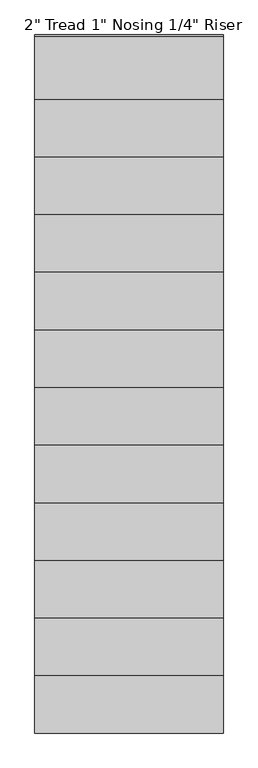
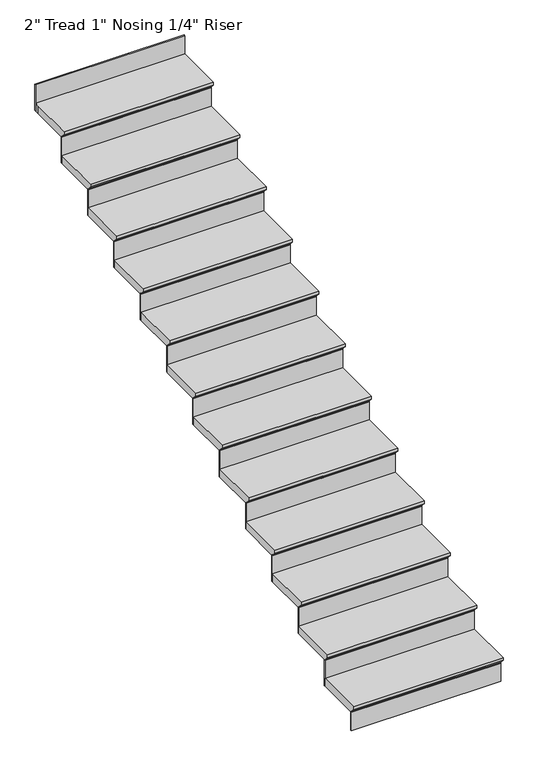
"""IFC4 building model written with IfcOpenShell, lengths in millimetres: stair flight geometry."""

from ifc_helpers import new_model, si_unit, origin, place, context, project, spatial, faceted_brep, source, transform, mapped, element, save


def stair_flight_74cd6fce(model_context):
    return source(origin(), model_context, "Body", "Brep", [
        faceted_brep([(-2703.0415084, 19841.9216096, 34528.9005799), (-2703.0415084, 19841.9216096, 34547.9505799), (-3617.4415084, 19841.9216096, 34547.9505799), (-3617.4415084, 19841.9216096, 34528.9005799), (-2703.0415084, 19867.3216096, 34503.5005799), (-3617.4415084, 19867.3216096, 34503.5005799), (-2703.0415084, 20146.7216096, 34547.9505799), (-3617.4415084, 20146.7216096, 34547.9505799), (-3617.4415084, 19867.3216096, 34497.1505799), (-3617.4415084, 20146.7216096, 34497.1505799), (-2703.0415084, 20146.7216096, 34497.1505799), (-2703.0415084, 19867.3216096, 34497.1505799)], [[[0, 1, 2, 3]], [[4, 0, 3, 5]], [[2, 1, 6, 7]], [[8, 9, 10, 11]], [[2, 7, 9, 8, 5, 3]], [[8, 11, 4, 5]], [[6, 1, 0, 4, 11, 10]], [[7, 6, 10, 9]]]),
        faceted_brep([(-2703.0415084, 19867.3216096, 34497.1505799), (-2703.0415084, 19867.3216096, 34378.6172466), (-2703.0415084, 19873.6716096, 34378.6172466), (-2703.0415084, 19873.6716096, 34497.1505799), (-3617.4415084, 19867.3216096, 34497.1505799), (-3617.4415084, 19873.6716096, 34497.1505799), (-3617.4415084, 19873.6716096, 34378.6172466), (-3617.4415084, 19867.3216096, 34378.6172466)], [[[0, 1, 2, 3]], [[4, 5, 6, 7]], [[1, 0, 4, 7]], [[2, 1, 7, 6]], [[3, 2, 6, 5]], [[0, 3, 5, 4]]]),
        faceted_brep([(-2703.0415084, 20146.7216096, 34666.4839133), (-2703.0415084, 20146.7216096, 34497.1505799), (-2703.0415084, 20153.0716096, 34497.1505799), (-2703.0415084, 20153.0716096, 34666.4839133), (-3617.4415084, 20146.7216096, 34666.4839133), (-3617.4415084, 20153.0716096, 34666.4839133), (-3617.4415084, 20153.0716096, 34497.1505799), (-3617.4415084, 20146.7216096, 34497.1505799)], [[[0, 1, 2, 3]], [[4, 5, 6, 7]], [[1, 0, 4, 7]], [[2, 1, 7, 6]], [[3, 2, 6, 5]], [[0, 3, 5, 4]]]),
        faceted_brep([(-3617.4415084, 20121.3216096, 34717.2839133), (-2703.0415084, 20121.3216096, 34717.2839133), (-2703.0415084, 20426.1216096, 34717.2839133), (-3617.4415084, 20426.1216096, 34717.2839133), (-3617.4415084, 20146.7216096, 34666.4839133), (-3617.4415084, 20426.1216096, 34666.4839133), (-2703.0415084, 20426.1216096, 34666.4839133), (-2703.0415084, 20146.7216096, 34666.4839133), (-3617.4415084, 20146.7216096, 34672.8339133), (-3617.4415084, 20121.3216096, 34698.2339133), (-2703.0415084, 20146.7216096, 34672.8339133), (-2703.0415084, 20121.3216096, 34698.2339133)], [[[0, 1, 2, 3]], [[4, 5, 6, 7]], [[0, 3, 5, 4, 8, 9]], [[4, 7, 10, 8]], [[2, 1, 11, 10, 7, 6]], [[3, 2, 6, 5]], [[11, 1, 0, 9]], [[10, 11, 9, 8]]]),
        faceted_brep([(-2703.0415084, 20426.1216096, 34835.8172466), (-2703.0415084, 20426.1216096, 34666.4839133), (-2703.0415084, 20432.4716096, 34666.4839133), (-2703.0415084, 20432.4716096, 34835.8172466), (-3617.4415084, 20426.1216096, 34835.8172466), (-3617.4415084, 20432.4716096, 34835.8172466), (-3617.4415084, 20432.4716096, 34666.4839133), (-3617.4415084, 20426.1216096, 34666.4839133)], [[[0, 1, 2, 3]], [[4, 5, 6, 7]], [[1, 0, 4, 7]], [[2, 1, 7, 6]], [[3, 2, 6, 5]], [[0, 3, 5, 4]]]),
        faceted_brep([(-3617.4415084, 20400.7216096, 34886.6172466), (-2703.0415084, 20400.7216096, 34886.6172466), (-2703.0415084, 20705.5216096, 34886.6172466), (-3617.4415084, 20705.5216096, 34886.6172466), (-3617.4415084, 20426.1216096, 34835.8172466), (-3617.4415084, 20705.5216096, 34835.8172466), (-2703.0415084, 20705.5216096, 34835.8172466), (-2703.0415084, 20426.1216096, 34835.8172466), (-3617.4415084, 20426.1216096, 34842.1672466), (-3617.4415084, 20400.7216096, 34867.5672466), (-2703.0415084, 20426.1216096, 34842.1672466), (-2703.0415084, 20400.7216096, 34867.5672466)], [[[0, 1, 2, 3]], [[4, 5, 6, 7]], [[0, 3, 5, 4, 8, 9]], [[4, 7, 10, 8]], [[2, 1, 11, 10, 7, 6]], [[3, 2, 6, 5]], [[11, 1, 0, 9]], [[10, 11, 9, 8]]]),
        faceted_brep([(-2703.0415084, 20705.5216096, 35005.1505799), (-2703.0415084, 20705.5216096, 34835.8172466), (-2703.0415084, 20711.8716096, 34835.8172466), (-2703.0415084, 20711.8716096, 35005.1505799), (-3617.4415084, 20705.5216096, 35005.1505799), (-3617.4415084, 20711.8716096, 35005.1505799), (-3617.4415084, 20711.8716096, 34835.8172466), (-3617.4415084, 20705.5216096, 34835.8172466)], [[[0, 1, 2, 3]], [[4, 5, 6, 7]], [[1, 0, 4, 7]], [[2, 1, 7, 6]], [[3, 2, 6, 5]], [[0, 3, 5, 4]]]),
        faceted_brep([(-3617.4415084, 20680.1216096, 35055.9505799), (-2703.0415084, 20680.1216096, 35055.9505799), (-2703.0415084, 20984.9216096, 35055.9505799), (-3617.4415084, 20984.9216096, 35055.9505799), (-3617.4415084, 20705.5216096, 35005.1505799), (-3617.4415084, 20984.9216096, 35005.1505799), (-2703.0415084, 20984.9216096, 35005.1505799), (-2703.0415084, 20705.5216096, 35005.1505799), (-3617.4415084, 20705.5216096, 35011.5005799), (-3617.4415084, 20680.1216096, 35036.9005799), (-2703.0415084, 20705.5216096, 35011.5005799), (-2703.0415084, 20680.1216096, 35036.9005799)], [[[0, 1, 2, 3]], [[4, 5, 6, 7]], [[0, 3, 5, 4, 8, 9]], [[4, 7, 10, 8]], [[2, 1, 11, 10, 7, 6]], [[3, 2, 6, 5]], [[11, 1, 0, 9]], [[10, 11, 9, 8]]]),
        faceted_brep([(-2703.0415084, 20984.9216096, 35174.4839133), (-2703.0415084, 20984.9216096, 35005.1505799), (-2703.0415084, 20991.2716096, 35005.1505799), (-2703.0415084, 20991.2716096, 35174.4839133), (-3617.4415084, 20984.9216096, 35174.4839133), (-3617.4415084, 20991.2716096, 35174.4839133), (-3617.4415084, 20991.2716096, 35005.1505799), (-3617.4415084, 20984.9216096, 35005.1505799)], [[[0, 1, 2, 3]], [[4, 5, 6, 7]], [[1, 0, 4, 7]], [[2, 1, 7, 6]], [[3, 2, 6, 5]], [[0, 3, 5, 4]]]),
        faceted_brep([(-3617.4415084, 20959.5216096, 35225.2839133), (-2703.0415084, 20959.5216096, 35225.2839133), (-2703.0415084, 21264.3216096, 35225.2839133), (-3617.4415084, 21264.3216096, 35225.2839133), (-3617.4415084, 20984.9216096, 35174.4839133), (-3617.4415084, 21264.3216096, 35174.4839133), (-2703.0415084, 21264.3216096, 35174.4839133), (-2703.0415084, 20984.9216096, 35174.4839133), (-3617.4415084, 20984.9216096, 35180.8339133), (-3617.4415084, 20959.5216096, 35206.2339133), (-2703.0415084, 20984.9216096, 35180.8339133), (-2703.0415084, 20959.5216096, 35206.2339133)], [[[0, 1, 2, 3]], [[4, 5, 6, 7]], [[0, 3, 5, 4, 8, 9]], [[4, 7, 10, 8]], [[2, 1, 11, 10, 7, 6]], [[3, 2, 6, 5]], [[11, 1, 0, 9]], [[10, 11, 9, 8]]]),
        faceted_brep([(-2703.0415084, 21264.3216096, 35343.8172466), (-2703.0415084, 21264.3216096, 35174.4839133), (-2703.0415084, 21270.6716096, 35174.4839133), (-2703.0415084, 21270.6716096, 35343.8172466), (-3617.4415084, 21264.3216096, 35343.8172466), (-3617.4415084, 21270.6716096, 35343.8172466), (-3617.4415084, 21270.6716096, 35174.4839133), (-3617.4415084, 21264.3216096, 35174.4839133)], [[[0, 1, 2, 3]], [[4, 5, 6, 7]], [[1, 0, 4, 7]], [[2, 1, 7, 6]], [[3, 2, 6, 5]], [[0, 3, 5, 4]]]),
        faceted_brep([(-3617.4415084, 21238.9216096, 35394.6172466), (-2703.0415084, 21238.9216096, 35394.6172466), (-2703.0415084, 21543.7216096, 35394.6172466), (-3617.4415084, 21543.7216096, 35394.6172466), (-3617.4415084, 21264.3216096, 35343.8172466), (-3617.4415084, 21543.7216096, 35343.8172466), (-2703.0415084, 21543.7216096, 35343.8172466), (-2703.0415084, 21264.3216096, 35343.8172466), (-3617.4415084, 21264.3216096, 35350.1672466), (-3617.4415084, 21238.9216096, 35375.5672466), (-2703.0415084, 21264.3216096, 35350.1672466), (-2703.0415084, 21238.9216096, 35375.5672466)], [[[0, 1, 2, 3]], [[4, 5, 6, 7]], [[0, 3, 5, 4, 8, 9]], [[4, 7, 10, 8]], [[2, 1, 11, 10, 7, 6]], [[3, 2, 6, 5]], [[11, 1, 0, 9]], [[10, 11, 9, 8]]]),
        faceted_brep([(-2703.0415084, 21543.7216096, 35513.1505799), (-2703.0415084, 21543.7216096, 35343.8172466), (-2703.0415084, 21550.0716096, 35343.8172466), (-2703.0415084, 21550.0716096, 35513.1505799), (-3617.4415084, 21543.7216096, 35513.1505799), (-3617.4415084, 21550.0716096, 35513.1505799), (-3617.4415084, 21550.0716096, 35343.8172466), (-3617.4415084, 21543.7216096, 35343.8172466)], [[[0, 1, 2, 3]], [[4, 5, 6, 7]], [[1, 0, 4, 7]], [[2, 1, 7, 6]], [[3, 2, 6, 5]], [[0, 3, 5, 4]]]),
        faceted_brep([(-3617.4415084, 21518.3216096, 35563.9505799), (-2703.0415084, 21518.3216096, 35563.9505799), (-2703.0415084, 21823.1216096, 35563.9505799), (-3617.4415084, 21823.1216096, 35563.9505799), (-3617.4415084, 21543.7216096, 35513.1505799), (-3617.4415084, 21823.1216096, 35513.1505799), (-2703.0415084, 21823.1216096, 35513.1505799), (-2703.0415084, 21543.7216096, 35513.1505799), (-3617.4415084, 21543.7216096, 35519.5005799), (-3617.4415084, 21518.3216096, 35544.9005799), (-2703.0415084, 21543.7216096, 35519.5005799), (-2703.0415084, 21518.3216096, 35544.9005799)], [[[0, 1, 2, 3]], [[4, 5, 6, 7]], [[0, 3, 5, 4, 8, 9]], [[4, 7, 10, 8]], [[2, 1, 11, 10, 7, 6]], [[3, 2, 6, 5]], [[11, 1, 0, 9]], [[10, 11, 9, 8]]]),
        faceted_brep([(-2703.0415084, 21823.1216096, 35682.4839133), (-2703.0415084, 21823.1216096, 35513.1505799), (-2703.0415084, 21829.4716096, 35513.1505799), (-2703.0415084, 21829.4716096, 35682.4839133), (-3617.4415084, 21823.1216096, 35682.4839133), (-3617.4415084, 21829.4716096, 35682.4839133), (-3617.4415084, 21829.4716096, 35513.1505799), (-3617.4415084, 21823.1216096, 35513.1505799)], [[[0, 1, 2, 3]], [[4, 5, 6, 7]], [[1, 0, 4, 7]], [[2, 1, 7, 6]], [[3, 2, 6, 5]], [[0, 3, 5, 4]]]),
        faceted_brep([(-3617.4415084, 21797.7216096, 35733.2839133), (-2703.0415084, 21797.7216096, 35733.2839133), (-2703.0415084, 22102.5216096, 35733.2839133), (-3617.4415084, 22102.5216096, 35733.2839133), (-3617.4415084, 21823.1216096, 35682.4839133), (-3617.4415084, 22102.5216096, 35682.4839133), (-2703.0415084, 22102.5216096, 35682.4839133), (-2703.0415084, 21823.1216096, 35682.4839133), (-3617.4415084, 21823.1216096, 35688.8339133), (-3617.4415084, 21797.7216096, 35714.2339133), (-2703.0415084, 21823.1216096, 35688.8339133), (-2703.0415084, 21797.7216096, 35714.2339133)], [[[0, 1, 2, 3]], [[4, 5, 6, 7]], [[0, 3, 5, 4, 8, 9]], [[4, 7, 10, 8]], [[2, 1, 11, 10, 7, 6]], [[3, 2, 6, 5]], [[11, 1, 0, 9]], [[10, 11, 9, 8]]]),
        faceted_brep([(-2703.0415084, 22102.5216096, 35851.8172466), (-2703.0415084, 22102.5216096, 35682.4839133), (-2703.0415084, 22108.8716096, 35682.4839133), (-2703.0415084, 22108.8716096, 35851.8172466), (-3617.4415084, 22102.5216096, 35851.8172466), (-3617.4415084, 22108.8716096, 35851.8172466), (-3617.4415084, 22108.8716096, 35682.4839133), (-3617.4415084, 22102.5216096, 35682.4839133)], [[[0, 1, 2, 3]], [[4, 5, 6, 7]], [[1, 0, 4, 7]], [[2, 1, 7, 6]], [[3, 2, 6, 5]], [[0, 3, 5, 4]]]),
        faceted_brep([(-3617.4415084, 22077.1216096, 35902.6172466), (-2703.0415084, 22077.1216096, 35902.6172466), (-2703.0415084, 22381.9216096, 35902.6172466), (-3617.4415084, 22381.9216096, 35902.6172466), (-3617.4415084, 22102.5216096, 35851.8172466), (-3617.4415084, 22381.9216096, 35851.8172466), (-2703.0415084, 22381.9216096, 35851.8172466), (-2703.0415084, 22102.5216096, 35851.8172466), (-3617.4415084, 22102.5216096, 35858.1672466), (-3617.4415084, 22077.1216096, 35883.5672466), (-2703.0415084, 22102.5216096, 35858.1672466), (-2703.0415084, 22077.1216096, 35883.5672466)], [[[0, 1, 2, 3]], [[4, 5, 6, 7]], [[0, 3, 5, 4, 8, 9]], [[4, 7, 10, 8]], [[2, 1, 11, 10, 7, 6]], [[3, 2, 6, 5]], [[11, 1, 0, 9]], [[10, 11, 9, 8]]]),
        faceted_brep([(-2703.0415084, 22381.9216096, 36021.1505799), (-2703.0415084, 22381.9216096, 35851.8172466), (-2703.0415084, 22388.2716096, 35851.8172466), (-2703.0415084, 22388.2716096, 36021.1505799), (-3617.4415084, 22381.9216096, 36021.1505799), (-3617.4415084, 22388.2716096, 36021.1505799), (-3617.4415084, 22388.2716096, 35851.8172466), (-3617.4415084, 22381.9216096, 35851.8172466)], [[[0, 1, 2, 3]], [[4, 5, 6, 7]], [[1, 0, 4, 7]], [[2, 1, 7, 6]], [[3, 2, 6, 5]], [[0, 3, 5, 4]]]),
        faceted_brep([(-3617.4415084, 22356.5216096, 36071.9505799), (-2703.0415084, 22356.5216096, 36071.9505799), (-2703.0415084, 22661.3216096, 36071.9505799), (-3617.4415084, 22661.3216096, 36071.9505799), (-3617.4415084, 22381.9216096, 36021.1505799), (-3617.4415084, 22661.3216096, 36021.1505799), (-2703.0415084, 22661.3216096, 36021.1505799), (-2703.0415084, 22381.9216096, 36021.1505799), (-3617.4415084, 22381.9216096, 36027.5005799), (-3617.4415084, 22356.5216096, 36052.9005799), (-2703.0415084, 22381.9216096, 36027.5005799), (-2703.0415084, 22356.5216096, 36052.9005799)], [[[0, 1, 2, 3]], [[4, 5, 6, 7]], [[0, 3, 5, 4, 8, 9]], [[4, 7, 10, 8]], [[2, 1, 11, 10, 7, 6]], [[3, 2, 6, 5]], [[11, 1, 0, 9]], [[10, 11, 9, 8]]]),
        faceted_brep([(-2703.0415084, 22661.3216096, 36190.4839133), (-2703.0415084, 22661.3216096, 36021.1505799), (-2703.0415084, 22667.6716096, 36021.1505799), (-2703.0415084, 22667.6716096, 36190.4839133), (-3617.4415084, 22661.3216096, 36190.4839133), (-3617.4415084, 22667.6716096, 36190.4839133), (-3617.4415084, 22667.6716096, 36021.1505799), (-3617.4415084, 22661.3216096, 36021.1505799)], [[[0, 1, 2, 3]], [[4, 5, 6, 7]], [[1, 0, 4, 7]], [[2, 1, 7, 6]], [[3, 2, 6, 5]], [[0, 3, 5, 4]]]),
        faceted_brep([(-3617.4415084, 22635.9216096, 36241.2839133), (-2703.0415084, 22635.9216096, 36241.2839133), (-2703.0415084, 22940.7216096, 36241.2839133), (-3617.4415084, 22940.7216096, 36241.2839133), (-3617.4415084, 22661.3216096, 36190.4839133), (-3617.4415084, 22940.7216096, 36190.4839133), (-2703.0415084, 22940.7216096, 36190.4839133), (-2703.0415084, 22661.3216096, 36190.4839133), (-3617.4415084, 22661.3216096, 36196.8339133), (-3617.4415084, 22635.9216096, 36222.2339133), (-2703.0415084, 22661.3216096, 36196.8339133), (-2703.0415084, 22635.9216096, 36222.2339133)], [[[0, 1, 2, 3]], [[4, 5, 6, 7]], [[0, 3, 5, 4, 8, 9]], [[4, 7, 10, 8]], [[2, 1, 11, 10, 7, 6]], [[3, 2, 6, 5]], [[11, 1, 0, 9]], [[10, 11, 9, 8]]]),
        faceted_brep([(-2703.0415084, 23220.1216096, 36529.1505799), (-2703.0415084, 23220.1216096, 36359.8172466), (-2703.0415084, 23226.4716096, 36359.8172466), (-2703.0415084, 23226.4716096, 36529.1505799), (-3617.4415084, 23220.1216096, 36529.1505799), (-3617.4415084, 23226.4716096, 36529.1505799), (-3617.4415084, 23226.4716096, 36359.8172466), (-3617.4415084, 23220.1216096, 36359.8172466)], [[[0, 1, 2, 3]], [[4, 5, 6, 7]], [[1, 0, 4, 7]], [[2, 1, 7, 6]], [[3, 2, 6, 5]], [[0, 3, 5, 4]]]),
        faceted_brep([(-2703.0415084, 22940.7216096, 36359.8172466), (-2703.0415084, 22940.7216096, 36190.4839133), (-2703.0415084, 22947.0716096, 36190.4839133), (-2703.0415084, 22947.0716096, 36359.8172466), (-3617.4415084, 22940.7216096, 36359.8172466), (-3617.4415084, 22947.0716096, 36359.8172466), (-3617.4415084, 22947.0716096, 36190.4839133), (-3617.4415084, 22940.7216096, 36190.4839133)], [[[0, 1, 2, 3]], [[4, 5, 6, 7]], [[1, 0, 4, 7]], [[2, 1, 7, 6]], [[3, 2, 6, 5]], [[0, 3, 5, 4]]]),
        faceted_brep([(-3617.4415084, 23220.1216096, 36410.6172466), (-3617.4415084, 23194.7216096, 36410.6172466), (-3617.4415084, 22915.3216096, 36410.6172466), (-2703.0415084, 22915.3216096, 36410.6172466), (-2703.0415084, 23220.1216096, 36410.6172466), (-3617.4415084, 23194.7216096, 36359.8172466), (-3617.4415084, 23220.1216096, 36359.8172466), (-2703.0415084, 23220.1216096, 36359.8172466), (-2703.0415084, 22940.7216096, 36359.8172466), (-3617.4415084, 22940.7216096, 36359.8172466), (-3617.4415084, 22940.7216096, 36366.1672466), (-3617.4415084, 22915.3216096, 36391.5672466), (-2703.0415084, 22940.7216096, 36366.1672466), (-2703.0415084, 22915.3216096, 36391.5672466)], [[[0, 1, 2, 3, 4]], [[5, 6, 7, 8, 9]], [[1, 0, 6, 5]], [[2, 1, 5, 9, 10, 11]], [[9, 8, 12, 10]], [[4, 3, 13, 12, 8, 7]], [[0, 4, 7, 6]], [[13, 3, 2, 11]], [[12, 13, 11, 10]]]),
    ])


if __name__ == "__main__":
    model = new_model("IFC4")
    model_context = context("Model", 3, world=origin())
    ifc_project = project(units=[si_unit("LENGTHUNIT", "METRE", prefix="MILLI")], contexts=[model_context])
    site = spatial("IfcSite", under=ifc_project)
    building = spatial("IfcBuilding", under=site)
    placement = place(None, origin())
    stair_flight_shape = stair_flight_74cd6fce(model_context)
    element("IfcStairFlight", 1, ObjectType="2\" Tread 1\" Nosing 1/4\" Riser", at=placement, inside=building, context=model_context, shape_type="MappedRepresentation", body=[
        mapped(stair_flight_shape, transform((0.0, 0.0, 0.0), x_axis=(1.0, 0.0, 0.0), y_axis=(0.0, 1.0, 0.0), z_axis=(0.0, 0.0, 1.0))),
    ])
    save(model, "model.ifc")
